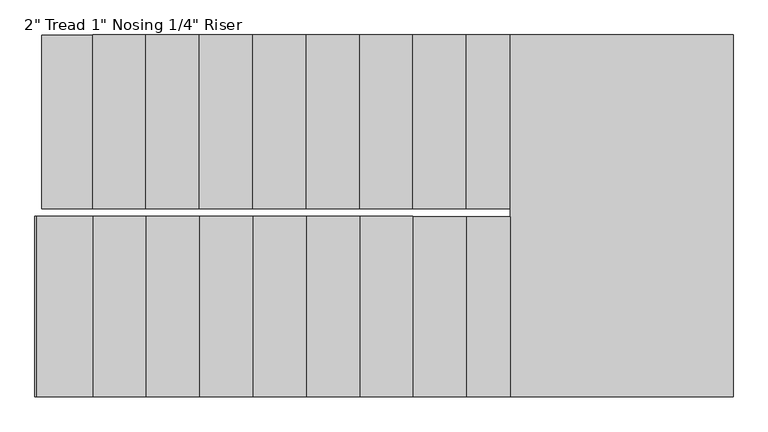
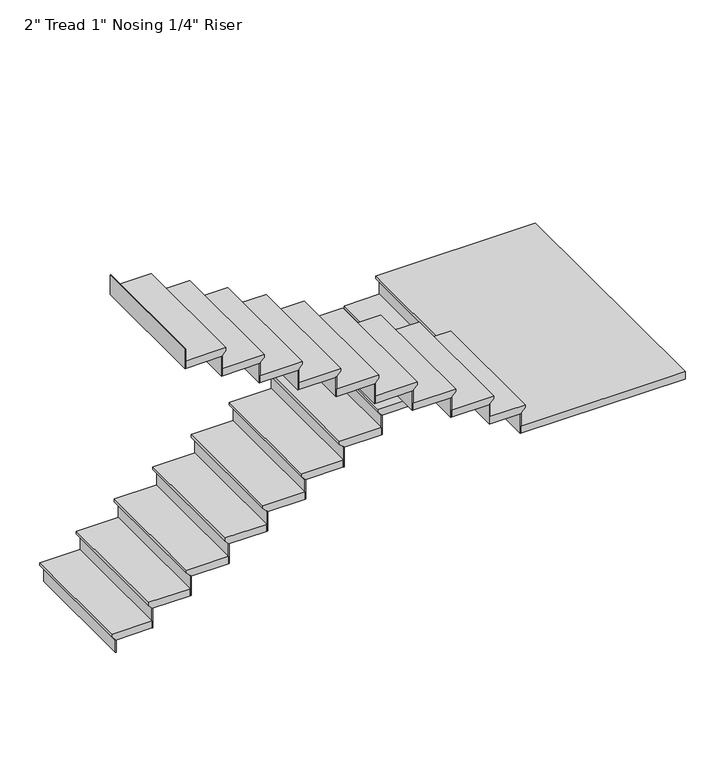
"""IFC4 building model written with IfcOpenShell, lengths in millimetres: stair flight geometry."""

from ifc_helpers import new_model, si_unit, origin, place, context, project, spatial, faceted_brep, source, transform, mapped, element, save


def stair_flight_00d6430a(model_context):
    return source(origin(), model_context, "Body", "Brep", [
        faceted_brep([(1537.1941283, 180.9547293, 118.11), (1537.1941283, 180.9547293, 137.16), (1537.1941283, 1006.4547293, 137.16), (1537.1941283, 1006.4547293, 118.11), (1562.5941283, 180.9547293, 92.71), (1562.5941283, 1006.4547293, 92.71), (1804.8381368, 180.9547293, 137.16), (1804.8381368, 1006.4547293, 137.16), (1562.5941283, 1006.4547293, 86.36), (1804.8381368, 1006.4547293, 86.36), (1804.8381368, 180.9547293, 86.36), (1562.5941283, 180.9547293, 86.36)], [[[0, 1, 2, 3]], [[4, 0, 3, 5]], [[2, 1, 6, 7]], [[8, 9, 10, 11]], [[2, 7, 9, 8, 5, 3]], [[8, 11, 4, 5]], [[6, 1, 0, 4, 11, 10]], [[7, 6, 10, 9]]]),
        faceted_brep([(1562.5941283, 180.9547293, 86.36), (1562.5941283, 180.9547293, 0.0), (1568.9441283, 180.9547293, 0.0), (1568.9441283, 180.9547293, 86.36), (1562.5941283, 1006.4547293, 86.36), (1568.9441283, 1006.4547293, 86.36), (1568.9441283, 1006.4547293, 0.0), (1562.5941283, 1006.4547293, 0.0)], [[[0, 1, 2, 3]], [[4, 5, 6, 7]], [[1, 0, 4, 7]], [[2, 1, 7, 6]], [[3, 2, 6, 5]], [[0, 3, 5, 4]]]),
        faceted_brep([(1804.8381368, 180.9547293, 223.52), (1804.8381368, 180.9547293, 86.36), (1811.1881368, 180.9547293, 86.36), (1811.1881368, 180.9547293, 223.52), (1804.8381368, 1006.4547293, 223.52), (1811.1881368, 1006.4547293, 223.52), (1811.1881368, 1006.4547293, 86.36), (1804.8381368, 1006.4547293, 86.36)], [[[0, 1, 2, 3]], [[4, 5, 6, 7]], [[1, 0, 4, 7]], [[2, 1, 7, 6]], [[3, 2, 6, 5]], [[0, 3, 5, 4]]]),
        faceted_brep([(1779.4381368, 1006.4547293, 274.32), (1779.4381368, 180.9547293, 274.32), (2058.8381368, 180.9547293, 274.32), (2058.8381368, 1006.4547293, 274.32), (1804.8381368, 1006.4547293, 223.52), (2058.8381368, 1006.4547293, 223.52), (2058.8381368, 180.9547293, 223.52), (1804.8381368, 180.9547293, 223.52), (1804.8381368, 1006.4547293, 229.87), (1779.4381368, 1006.4547293, 255.27), (1804.8381368, 180.9547293, 229.87), (1779.4381368, 180.9547293, 255.27)], [[[0, 1, 2, 3]], [[4, 5, 6, 7]], [[0, 3, 5, 4, 8, 9]], [[4, 7, 10, 8]], [[2, 1, 11, 10, 7, 6]], [[3, 2, 6, 5]], [[11, 1, 0, 9]], [[10, 11, 9, 8]]]),
        faceted_brep([(2058.8381368, 180.9547293, 360.68), (2058.8381368, 180.9547293, 223.52), (2065.1881368, 180.9547293, 223.52), (2065.1881368, 180.9547293, 360.68), (2058.8381368, 1006.4547293, 360.68), (2065.1881368, 1006.4547293, 360.68), (2065.1881368, 1006.4547293, 223.52), (2058.8381368, 1006.4547293, 223.52)], [[[0, 1, 2, 3]], [[4, 5, 6, 7]], [[1, 0, 4, 7]], [[2, 1, 7, 6]], [[3, 2, 6, 5]], [[0, 3, 5, 4]]]),
        faceted_brep([(2033.4381368, 1006.4547293, 411.48), (2033.4381368, 180.9547293, 411.48), (2312.8381368, 180.9547293, 411.48), (2312.8381368, 1006.4547293, 411.48), (2058.8381368, 1006.4547293, 360.68), (2312.8381368, 1006.4547293, 360.68), (2312.8381368, 180.9547293, 360.68), (2058.8381368, 180.9547293, 360.68), (2058.8381368, 1006.4547293, 367.03), (2033.4381368, 1006.4547293, 392.43), (2058.8381368, 180.9547293, 367.03), (2033.4381368, 180.9547293, 392.43)], [[[0, 1, 2, 3]], [[4, 5, 6, 7]], [[0, 3, 5, 4, 8, 9]], [[4, 7, 10, 8]], [[2, 1, 11, 10, 7, 6]], [[3, 2, 6, 5]], [[11, 1, 0, 9]], [[10, 11, 9, 8]]]),
        faceted_brep([(2312.8381368, 180.9547293, 497.84), (2312.8381368, 180.9547293, 360.68), (2319.1881368, 180.9547293, 360.68), (2319.1881368, 180.9547293, 497.84), (2312.8381368, 1006.4547293, 497.84), (2319.1881368, 1006.4547293, 497.84), (2319.1881368, 1006.4547293, 360.68), (2312.8381368, 1006.4547293, 360.68)], [[[0, 1, 2, 3]], [[4, 5, 6, 7]], [[1, 0, 4, 7]], [[2, 1, 7, 6]], [[3, 2, 6, 5]], [[0, 3, 5, 4]]]),
        faceted_brep([(2287.4381368, 1006.4547293, 548.64), (2287.4381368, 180.9547293, 548.64), (2566.8381368, 180.9547293, 548.64), (2566.8381368, 1006.4547293, 548.64), (2312.8381368, 1006.4547293, 497.84), (2566.8381368, 1006.4547293, 497.84), (2566.8381368, 180.9547293, 497.84), (2312.8381368, 180.9547293, 497.84), (2312.8381368, 1006.4547293, 504.19), (2287.4381368, 1006.4547293, 529.59), (2312.8381368, 180.9547293, 504.19), (2287.4381368, 180.9547293, 529.59)], [[[0, 1, 2, 3]], [[4, 5, 6, 7]], [[0, 3, 5, 4, 8, 9]], [[4, 7, 10, 8]], [[2, 1, 11, 10, 7, 6]], [[3, 2, 6, 5]], [[11, 1, 0, 9]], [[10, 11, 9, 8]]]),
        faceted_brep([(2566.8381368, 180.9547293, 635.0), (2566.8381368, 180.9547293, 497.84), (2573.1881368, 180.9547293, 497.84), (2573.1881368, 180.9547293, 635.0), (2566.8381368, 1006.4547293, 635.0), (2573.1881368, 1006.4547293, 635.0), (2573.1881368, 1006.4547293, 497.84), (2566.8381368, 1006.4547293, 497.84)], [[[0, 1, 2, 3]], [[4, 5, 6, 7]], [[1, 0, 4, 7]], [[2, 1, 7, 6]], [[3, 2, 6, 5]], [[0, 3, 5, 4]]]),
        faceted_brep([(2541.4381368, 1006.4547293, 685.8), (2541.4381368, 180.9547293, 685.8), (2820.8381368, 180.9547293, 685.8), (2820.8381368, 1006.4547293, 685.8), (2566.8381368, 1006.4547293, 635.0), (2820.8381368, 1006.4547293, 635.0), (2820.8381368, 180.9547293, 635.0), (2566.8381368, 180.9547293, 635.0), (2566.8381368, 1006.4547293, 641.35), (2541.4381368, 1006.4547293, 666.75), (2566.8381368, 180.9547293, 641.35), (2541.4381368, 180.9547293, 666.75)], [[[0, 1, 2, 3]], [[4, 5, 6, 7]], [[0, 3, 5, 4, 8, 9]], [[4, 7, 10, 8]], [[2, 1, 11, 10, 7, 6]], [[3, 2, 6, 5]], [[11, 1, 0, 9]], [[10, 11, 9, 8]]]),
        faceted_brep([(2820.8381368, 180.9547293, 772.16), (2820.8381368, 180.9547293, 635.0), (2827.1881368, 180.9547293, 635.0), (2827.1881368, 180.9547293, 772.16), (2820.8381368, 1006.4547293, 772.16), (2827.1881368, 1006.4547293, 772.16), (2827.1881368, 1006.4547293, 635.0), (2820.8381368, 1006.4547293, 635.0)], [[[0, 1, 2, 3]], [[4, 5, 6, 7]], [[1, 0, 4, 7]], [[2, 1, 7, 6]], [[3, 2, 6, 5]], [[0, 3, 5, 4]]]),
        faceted_brep([(2795.4381368, 1006.4547293, 822.96), (2795.4381368, 180.9547293, 822.96), (3074.8381368, 180.9547293, 822.96), (3074.8381368, 1006.4547293, 822.96), (2820.8381368, 1006.4547293, 772.16), (3074.8381368, 1006.4547293, 772.16), (3074.8381368, 180.9547293, 772.16), (2820.8381368, 180.9547293, 772.16), (2820.8381368, 1006.4547293, 778.51), (2795.4381368, 1006.4547293, 803.91), (2820.8381368, 180.9547293, 778.51), (2795.4381368, 180.9547293, 803.91)], [[[0, 1, 2, 3]], [[4, 5, 6, 7]], [[0, 3, 5, 4, 8, 9]], [[4, 7, 10, 8]], [[2, 1, 11, 10, 7, 6]], [[3, 2, 6, 5]], [[11, 1, 0, 9]], [[10, 11, 9, 8]]]),
        faceted_brep([(3074.8381368, 180.9547293, 909.32), (3074.8381368, 180.9547293, 772.16), (3081.1881368, 180.9547293, 772.16), (3081.1881368, 180.9547293, 909.32), (3074.8381368, 1006.4547293, 909.32), (3081.1881368, 1006.4547293, 909.32), (3081.1881368, 1006.4547293, 772.16), (3074.8381368, 1006.4547293, 772.16)], [[[0, 1, 2, 3]], [[4, 5, 6, 7]], [[1, 0, 4, 7]], [[2, 1, 7, 6]], [[3, 2, 6, 5]], [[0, 3, 5, 4]]]),
        faceted_brep([(3049.4381368, 1006.4547293, 960.12), (3049.4381368, 180.9547293, 960.12), (3328.8381368, 180.9547293, 960.12), (3328.8381368, 1006.4547293, 960.12), (3074.8381368, 1006.4547293, 909.32), (3328.8381368, 1006.4547293, 909.32), (3328.8381368, 180.9547293, 909.32), (3074.8381368, 180.9547293, 909.32), (3074.8381368, 1006.4547293, 915.67), (3049.4381368, 1006.4547293, 941.07), (3074.8381368, 180.9547293, 915.67), (3049.4381368, 180.9547293, 941.07)], [[[0, 1, 2, 3]], [[4, 5, 6, 7]], [[0, 3, 5, 4, 8, 9]], [[4, 7, 10, 8]], [[2, 1, 11, 10, 7, 6]], [[3, 2, 6, 5]], [[11, 1, 0, 9]], [[10, 11, 9, 8]]]),
        faceted_brep([(3328.8381368, 180.9547293, 1046.48), (3328.8381368, 180.9547293, 909.32), (3335.1881368, 180.9547293, 909.32), (3335.1881368, 180.9547293, 1046.48), (3328.8381368, 1006.4547293, 1046.48), (3335.1881368, 1006.4547293, 1046.48), (3335.1881368, 1006.4547293, 909.32), (3328.8381368, 1006.4547293, 909.32)], [[[0, 1, 2, 3]], [[4, 5, 6, 7]], [[1, 0, 4, 7]], [[2, 1, 7, 6]], [[3, 2, 6, 5]], [[0, 3, 5, 4]]]),
        faceted_brep([(3303.4381368, 1006.4547293, 1097.28), (3303.4381368, 180.9547293, 1097.28), (3582.8381368, 180.9547293, 1097.28), (3582.8381368, 1006.4547293, 1097.28), (3328.8381368, 1006.4547293, 1046.48), (3582.8381368, 1006.4547293, 1046.48), (3582.8381368, 180.9547293, 1046.48), (3328.8381368, 180.9547293, 1046.48), (3328.8381368, 1006.4547293, 1052.83), (3303.4381368, 1006.4547293, 1078.23), (3328.8381368, 180.9547293, 1052.83), (3303.4381368, 180.9547293, 1078.23)], [[[0, 1, 2, 3]], [[4, 5, 6, 7]], [[0, 3, 5, 4, 8, 9]], [[4, 7, 10, 8]], [[2, 1, 11, 10, 7, 6]], [[3, 2, 6, 5]], [[11, 1, 0, 9]], [[10, 11, 9, 8]]]),
        faceted_brep([(3582.8381368, 180.9547293, 1183.64), (3582.8381368, 180.9547293, 1046.48), (3589.1881368, 180.9547293, 1046.48), (3589.1881368, 180.9547293, 1183.64), (3582.8381368, 1006.4547293, 1183.64), (3589.1881368, 1006.4547293, 1183.64), (3589.1881368, 1006.4547293, 1046.48), (3582.8381368, 1006.4547293, 1046.48)], [[[0, 1, 2, 3]], [[4, 5, 6, 7]], [[1, 0, 4, 7]], [[2, 1, 7, 6]], [[3, 2, 6, 5]], [[0, 3, 5, 4]]]),
        faceted_brep([(3557.4381368, 1006.4547293, 1234.44), (3557.4381368, 180.9547293, 1234.44), (3791.2648053, 180.9547293, 1234.44), (3791.2648053, 1006.4547293, 1234.44), (3582.8381368, 1006.4547293, 1183.64), (3791.2648053, 1006.4547293, 1183.64), (3791.2648053, 180.9547293, 1183.64), (3582.8381368, 180.9547293, 1183.64), (3582.8381368, 1006.4547293, 1189.99), (3557.4381368, 1006.4547293, 1215.39), (3582.8381368, 180.9547293, 1189.99), (3557.4381368, 180.9547293, 1215.39)], [[[0, 1, 2, 3]], [[4, 5, 6, 7]], [[0, 3, 5, 4, 8, 9]], [[4, 7, 10, 8]], [[2, 1, 11, 10, 7, 6]], [[3, 2, 6, 5]], [[11, 1, 0, 9]], [[10, 11, 9, 8]]]),
        faceted_brep([(3791.2648053, 180.9547293, 1320.8), (3791.2648053, 180.9547293, 1183.64), (3797.6148053, 180.9547293, 1183.64), (3797.6148053, 180.9547293, 1320.8), (3791.2648053, 1006.4547293, 1320.8), (3797.6148053, 1006.4547293, 1320.8), (3797.6148053, 1006.4547293, 1183.64), (3791.2648053, 1006.4547293, 1183.64)], [[[0, 1, 2, 3]], [[4, 5, 6, 7]], [[1, 0, 4, 7]], [[2, 1, 7, 6]], [[3, 2, 6, 5]], [[0, 3, 5, 4]]]),
        faceted_brep([(3740.4648053, -714.2964201, 1371.6), (4826.4941283, -714.2964201, 1371.6), (4826.4941283, 1006.4547293, 1371.6), (3765.8648053, 1006.4547293, 1371.6), (3765.8648053, 142.8547293, 1371.6), (3740.4648053, 142.8547293, 1371.6), (4826.4941283, -714.2964201, 1320.8), (3740.4648053, -714.2964201, 1320.8), (3740.4648053, 142.8547293, 1320.8), (3765.8648053, 142.8547293, 1320.8), (3765.8648053, 180.9547293, 1320.8), (3791.2648053, 180.9547293, 1320.8), (3791.2648053, 1006.4547293, 1320.8), (4826.4941283, 1006.4547293, 1320.8), (3791.2648053, 1006.4547293, 1327.15), (3765.8648053, 1006.4547293, 1352.55), (3791.2648053, 180.9547293, 1327.15), (3765.8648053, 180.9547293, 1352.55)], [[[0, 1, 2, 3, 4, 5]], [[6, 7, 8, 9, 10, 11, 12, 13]], [[1, 0, 7, 6]], [[2, 1, 6, 13]], [[3, 2, 13, 12, 14, 15]], [[12, 11, 16, 14]], [[11, 10, 17, 16]], [[4, 3, 15, 17, 10, 9]], [[5, 4, 9, 8]], [[0, 5, 8, 7]], [[15, 14, 16, 17]]]),
        faceted_brep([(3740.4648053, 142.8547293, 1457.96), (3740.4648053, 142.8547293, 1320.8), (3734.1148053, 142.8547293, 1320.8), (3734.1148053, 142.8547293, 1457.96), (3740.4648053, -714.2964201, 1457.96), (3734.1148053, -714.2964201, 1457.96), (3734.1148053, -714.2964201, 1320.8), (3740.4648053, -714.2964201, 1320.8)], [[[0, 1, 2, 3]], [[4, 5, 6, 7]], [[1, 0, 4, 7]], [[2, 1, 7, 6]], [[3, 2, 6, 5]], [[0, 3, 5, 4]]]),
        faceted_brep([(3765.8648053, -714.2964201, 1508.76), (3765.8648053, 142.8547293, 1508.76), (3532.0381368, 142.8547293, 1508.76), (3532.0381368, -714.2964201, 1508.76), (3740.4648053, -714.2964201, 1457.96), (3532.0381368, -714.2964201, 1457.96), (3532.0381368, 142.8547293, 1457.96), (3740.4648053, 142.8547293, 1457.96), (3740.4648053, -714.2964201, 1464.31), (3765.8648053, -714.2964201, 1489.71), (3740.4648053, 142.8547293, 1464.31), (3765.8648053, 142.8547293, 1489.71)], [[[0, 1, 2, 3]], [[4, 5, 6, 7]], [[0, 3, 5, 4, 8, 9]], [[4, 7, 10, 8]], [[2, 1, 11, 10, 7, 6]], [[3, 2, 6, 5]], [[11, 1, 0, 9]], [[10, 11, 9, 8]]]),
        faceted_brep([(3532.0381368, 142.8547293, 1595.12), (3532.0381368, 142.8547293, 1457.96), (3525.6881368, 142.8547293, 1457.96), (3525.6881368, 142.8547293, 1595.12), (3532.0381368, -714.2964201, 1595.12), (3525.6881368, -714.2964201, 1595.12), (3525.6881368, -714.2964201, 1457.96), (3532.0381368, -714.2964201, 1457.96)], [[[0, 1, 2, 3]], [[4, 5, 6, 7]], [[1, 0, 4, 7]], [[2, 1, 7, 6]], [[3, 2, 6, 5]], [[0, 3, 5, 4]]]),
        faceted_brep([(3557.4381368, -714.2964201, 1645.92), (3557.4381368, 142.8547293, 1645.92), (3278.0381368, 142.8547293, 1645.92), (3278.0381368, -714.2964201, 1645.92), (3532.0381368, -714.2964201, 1595.12), (3278.0381368, -714.2964201, 1595.12), (3278.0381368, 142.8547293, 1595.12), (3532.0381368, 142.8547293, 1595.12), (3532.0381368, -714.2964201, 1601.47), (3557.4381368, -714.2964201, 1626.87), (3532.0381368, 142.8547293, 1601.47), (3557.4381368, 142.8547293, 1626.87)], [[[0, 1, 2, 3]], [[4, 5, 6, 7]], [[0, 3, 5, 4, 8, 9]], [[4, 7, 10, 8]], [[2, 1, 11, 10, 7, 6]], [[3, 2, 6, 5]], [[11, 1, 0, 9]], [[10, 11, 9, 8]]]),
        faceted_brep([(3278.0381368, 142.8547293, 1732.28), (3278.0381368, 142.8547293, 1595.12), (3271.6881368, 142.8547293, 1595.12), (3271.6881368, 142.8547293, 1732.28), (3278.0381368, -714.2964201, 1732.28), (3271.6881368, -714.2964201, 1732.28), (3271.6881368, -714.2964201, 1595.12), (3278.0381368, -714.2964201, 1595.12)], [[[0, 1, 2, 3]], [[4, 5, 6, 7]], [[1, 0, 4, 7]], [[2, 1, 7, 6]], [[3, 2, 6, 5]], [[0, 3, 5, 4]]]),
        faceted_brep([(3303.4381368, -714.2964201, 1783.08), (3303.4381368, 142.8547293, 1783.08), (3024.0381368, 142.8547293, 1783.08), (3024.0381368, -714.2964201, 1783.08), (3278.0381368, -714.2964201, 1732.28), (3024.0381368, -714.2964201, 1732.28), (3024.0381368, 142.8547293, 1732.28), (3278.0381368, 142.8547293, 1732.28), (3278.0381368, -714.2964201, 1738.63), (3303.4381368, -714.2964201, 1764.03), (3278.0381368, 142.8547293, 1738.63), (3303.4381368, 142.8547293, 1764.03)], [[[0, 1, 2, 3]], [[4, 5, 6, 7]], [[0, 3, 5, 4, 8, 9]], [[4, 7, 10, 8]], [[2, 1, 11, 10, 7, 6]], [[3, 2, 6, 5]], [[11, 1, 0, 9]], [[10, 11, 9, 8]]]),
        faceted_brep([(3024.0381368, 142.8547293, 1869.44), (3024.0381368, 142.8547293, 1732.28), (3017.6881368, 142.8547293, 1732.28), (3017.6881368, 142.8547293, 1869.44), (3024.0381368, -714.2964201, 1869.44), (3017.6881368, -714.2964201, 1869.44), (3017.6881368, -714.2964201, 1732.28), (3024.0381368, -714.2964201, 1732.28)], [[[0, 1, 2, 3]], [[4, 5, 6, 7]], [[1, 0, 4, 7]], [[2, 1, 7, 6]], [[3, 2, 6, 5]], [[0, 3, 5, 4]]]),
        faceted_brep([(3049.4381368, -714.2964201, 1920.24), (3049.4381368, 142.8547293, 1920.24), (2770.0381368, 142.8547293, 1920.24), (2770.0381368, -714.2964201, 1920.24), (3024.0381368, -714.2964201, 1869.44), (2770.0381368, -714.2964201, 1869.44), (2770.0381368, 142.8547293, 1869.44), (3024.0381368, 142.8547293, 1869.44), (3024.0381368, -714.2964201, 1875.79), (3049.4381368, -714.2964201, 1901.19), (3024.0381368, 142.8547293, 1875.79), (3049.4381368, 142.8547293, 1901.19)], [[[0, 1, 2, 3]], [[4, 5, 6, 7]], [[0, 3, 5, 4, 8, 9]], [[4, 7, 10, 8]], [[2, 1, 11, 10, 7, 6]], [[3, 2, 6, 5]], [[11, 1, 0, 9]], [[10, 11, 9, 8]]]),
        faceted_brep([(2770.0381368, 142.8547293, 2006.6), (2770.0381368, 142.8547293, 1869.44), (2763.6881368, 142.8547293, 1869.44), (2763.6881368, 142.8547293, 2006.6), (2770.0381368, -714.2964201, 2006.6), (2763.6881368, -714.2964201, 2006.6), (2763.6881368, -714.2964201, 1869.44), (2770.0381368, -714.2964201, 1869.44)], [[[0, 1, 2, 3]], [[4, 5, 6, 7]], [[1, 0, 4, 7]], [[2, 1, 7, 6]], [[3, 2, 6, 5]], [[0, 3, 5, 4]]]),
        faceted_brep([(2795.4381368, -714.2964201, 2057.4), (2795.4381368, 142.8547293, 2057.4), (2516.0381368, 142.8547293, 2057.4), (2516.0381368, -714.2964201, 2057.4), (2770.0381368, -714.2964201, 2006.6), (2516.0381368, -714.2964201, 2006.6), (2516.0381368, 142.8547293, 2006.6), (2770.0381368, 142.8547293, 2006.6), (2770.0381368, -714.2964201, 2012.95), (2795.4381368, -714.2964201, 2038.35), (2770.0381368, 142.8547293, 2012.95), (2795.4381368, 142.8547293, 2038.35)], [[[0, 1, 2, 3]], [[4, 5, 6, 7]], [[0, 3, 5, 4, 8, 9]], [[4, 7, 10, 8]], [[2, 1, 11, 10, 7, 6]], [[3, 2, 6, 5]], [[11, 1, 0, 9]], [[10, 11, 9, 8]]]),
        faceted_brep([(2516.0381368, 142.8547293, 2143.76), (2516.0381368, 142.8547293, 2006.6), (2509.6881368, 142.8547293, 2006.6), (2509.6881368, 142.8547293, 2143.76), (2516.0381368, -714.2964201, 2143.76), (2509.6881368, -714.2964201, 2143.76), (2509.6881368, -714.2964201, 2006.6), (2516.0381368, -714.2964201, 2006.6)], [[[0, 1, 2, 3]], [[4, 5, 6, 7]], [[1, 0, 4, 7]], [[2, 1, 7, 6]], [[3, 2, 6, 5]], [[0, 3, 5, 4]]]),
        faceted_brep([(2541.4381368, -714.2964201, 2194.56), (2541.4381368, 142.8547293, 2194.56), (2262.0381368, 142.8547293, 2194.56), (2262.0381368, -714.2964201, 2194.56), (2516.0381368, -714.2964201, 2143.76), (2262.0381368, -714.2964201, 2143.76), (2262.0381368, 142.8547293, 2143.76), (2516.0381368, 142.8547293, 2143.76), (2516.0381368, -714.2964201, 2150.11), (2541.4381368, -714.2964201, 2175.51), (2516.0381368, 142.8547293, 2150.11), (2541.4381368, 142.8547293, 2175.51)], [[[0, 1, 2, 3]], [[4, 5, 6, 7]], [[0, 3, 5, 4, 8, 9]], [[4, 7, 10, 8]], [[2, 1, 11, 10, 7, 6]], [[3, 2, 6, 5]], [[11, 1, 0, 9]], [[10, 11, 9, 8]]]),
        faceted_brep([(2262.0381368, 142.8547293, 2280.92), (2262.0381368, 142.8547293, 2143.76), (2255.6881368, 142.8547293, 2143.76), (2255.6881368, 142.8547293, 2280.92), (2262.0381368, -714.2964201, 2280.92), (2255.6881368, -714.2964201, 2280.92), (2255.6881368, -714.2964201, 2143.76), (2262.0381368, -714.2964201, 2143.76)], [[[0, 1, 2, 3]], [[4, 5, 6, 7]], [[1, 0, 4, 7]], [[2, 1, 7, 6]], [[3, 2, 6, 5]], [[0, 3, 5, 4]]]),
        faceted_brep([(2287.4381368, -714.2964201, 2331.72), (2287.4381368, 142.8547293, 2331.72), (2008.0381368, 142.8547293, 2331.72), (2008.0381368, -714.2964201, 2331.72), (2262.0381368, -714.2964201, 2280.92), (2008.0381368, -714.2964201, 2280.92), (2008.0381368, 142.8547293, 2280.92), (2262.0381368, 142.8547293, 2280.92), (2262.0381368, -714.2964201, 2287.27), (2287.4381368, -714.2964201, 2312.67), (2262.0381368, 142.8547293, 2287.27), (2287.4381368, 142.8547293, 2312.67)], [[[0, 1, 2, 3]], [[4, 5, 6, 7]], [[0, 3, 5, 4, 8, 9]], [[4, 7, 10, 8]], [[2, 1, 11, 10, 7, 6]], [[3, 2, 6, 5]], [[11, 1, 0, 9]], [[10, 11, 9, 8]]]),
        faceted_brep([(2008.0381368, 142.8547293, 2418.08), (2008.0381368, 142.8547293, 2280.92), (2001.6881368, 142.8547293, 2280.92), (2001.6881368, 142.8547293, 2418.08), (2008.0381368, -714.2964201, 2418.08), (2001.6881368, -714.2964201, 2418.08), (2001.6881368, -714.2964201, 2280.92), (2008.0381368, -714.2964201, 2280.92)], [[[0, 1, 2, 3]], [[4, 5, 6, 7]], [[1, 0, 4, 7]], [[2, 1, 7, 6]], [[3, 2, 6, 5]], [[0, 3, 5, 4]]]),
        faceted_brep([(2033.4381368, -714.2964201, 2468.88), (2033.4381368, 142.8547293, 2468.88), (1754.0381368, 142.8547293, 2468.88), (1754.0381368, -714.2964201, 2468.88), (2008.0381368, -714.2964201, 2418.08), (1754.0381368, -714.2964201, 2418.08), (1754.0381368, 142.8547293, 2418.08), (2008.0381368, 142.8547293, 2418.08), (2008.0381368, -714.2964201, 2424.43), (2033.4381368, -714.2964201, 2449.83), (2008.0381368, 142.8547293, 2424.43), (2033.4381368, 142.8547293, 2449.83)], [[[0, 1, 2, 3]], [[4, 5, 6, 7]], [[0, 3, 5, 4, 8, 9]], [[4, 7, 10, 8]], [[2, 1, 11, 10, 7, 6]], [[3, 2, 6, 5]], [[11, 1, 0, 9]], [[10, 11, 9, 8]]]),
        faceted_brep([(1754.0381368, 142.8547293, 2555.24), (1754.0381368, 142.8547293, 2418.08), (1747.6881368, 142.8547293, 2418.08), (1747.6881368, 142.8547293, 2555.24), (1754.0381368, -714.2964201, 2555.24), (1747.6881368, -714.2964201, 2555.24), (1747.6881368, -714.2964201, 2418.08), (1754.0381368, -714.2964201, 2418.08)], [[[0, 1, 2, 3]], [[4, 5, 6, 7]], [[1, 0, 4, 7]], [[2, 1, 7, 6]], [[3, 2, 6, 5]], [[0, 3, 5, 4]]]),
        faceted_brep([(1511.7941283, 142.8547293, 2692.4), (1511.7941283, 142.8547293, 2555.24), (1505.4441283, 142.8547293, 2555.24), (1505.4441283, 142.8547293, 2692.4), (1511.7941283, -714.2964201, 2692.4), (1505.4441283, -714.2964201, 2692.4), (1505.4441283, -714.2964201, 2555.24), (1511.7941283, -714.2964201, 2555.24)], [[[0, 1, 2, 3]], [[4, 5, 6, 7]], [[1, 0, 4, 7]], [[2, 1, 7, 6]], [[3, 2, 6, 5]], [[0, 3, 5, 4]]]),
        faceted_brep([(1779.4381368, -714.2964201, 2606.04), (1779.4381368, 142.8547293, 2606.04), (1511.7941283, 142.8547293, 2606.04), (1511.7941283, -714.2964201, 2606.04), (1754.0381368, -714.2964201, 2555.24), (1511.7941283, -714.2964201, 2555.24), (1511.7941283, 142.8547293, 2555.24), (1754.0381368, 142.8547293, 2555.24), (1754.0381368, -714.2964201, 2561.59), (1779.4381368, -714.2964201, 2586.99), (1754.0381368, 142.8547293, 2561.59), (1779.4381368, 142.8547293, 2586.99)], [[[0, 1, 2, 3]], [[4, 5, 6, 7]], [[0, 3, 5, 4, 8, 9]], [[4, 7, 10, 8]], [[2, 1, 11, 10, 7, 6]], [[3, 2, 6, 5]], [[11, 1, 0, 9]], [[10, 11, 9, 8]]]),
    ])


if __name__ == "__main__":
    model = new_model("IFC4")
    model_context = context("Model", 3, world=origin())
    ifc_project = project(units=[si_unit("LENGTHUNIT", "METRE", prefix="MILLI")], contexts=[model_context])
    site = spatial("IfcSite", under=ifc_project)
    building = spatial("IfcBuilding", under=site)
    placement = place(None, origin())
    stair_flight_shape = stair_flight_00d6430a(model_context)
    element("IfcStairFlight", 1, ObjectType="2\" Tread 1\" Nosing 1/4\" Riser", at=placement, inside=building, context=model_context, shape_type="MappedRepresentation", body=[
        mapped(stair_flight_shape, transform((0.0, 0.0, 0.0), x_axis=(1.0, 0.0, 0.0), y_axis=(0.0, 1.0, 0.0), z_axis=(0.0, 0.0, 1.0))),
    ])
    save(model, "model.ifc")
